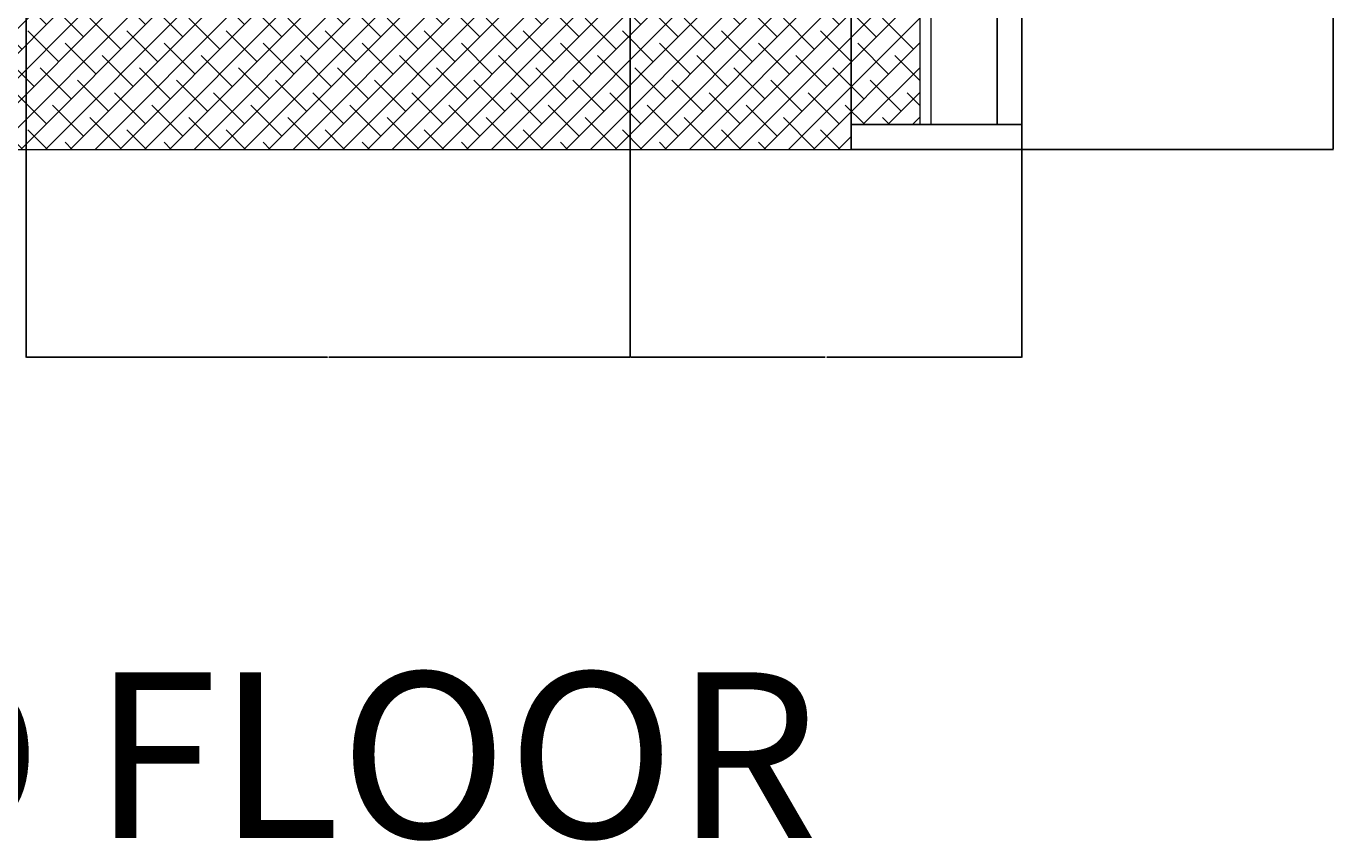
# Model space of a CAD drawing. Units: inches. Extents: x -4843 to -3402, y -164 to 3629.
# Tile 2 of 22: x -4303 to -3829, y -164 to 131. Entities that reach past the tile are written whole.
import ezdxf

# ---------------------------------------------------------------- set-up
doc = ezdxf.new("R2010")
doc.units = ezdxf.units.IN
for name, color, linetype, lineweight in [('A-ANNO-DIMS', 2, 'Continuous', 18), ('A-ANNO-TEXT', 7, 'Continuous', 25), ('C-PROP', 7, 'Continuous', 25), ('C-PVMT', 7, 'Continuous', 18), ('L-PLNT-EDGE', 7, 'Continuous', 18)]:
    doc.layers.add(name, color=color, linetype=linetype, lineweight=lineweight)
doc.layers.add('C-PVMT-PATT', color=9, linetype='Continuous', lineweight=13, true_color=0xc7c8ca)
doc.styles.get("Standard").update_dxf_attribs({"font": 'arial.ttf'})
doc.dimstyles.get("Standard").update_dxf_attribs({"dimtxt": 0.18, "dimasz": 0.18, "dimexe": 0.18, "dimexo": 0.0625, "dimgap": 0.09, "dimtad": 0, "dimtih": 1, "dimtoh": 1, "dimdec": 4, "dimzin": 0, "dimdsep": 46, "dimtxsty": 'Standard', "dimcen": 0.09, "dimadec": 0, "dimazin": 0, "dimtfac": 1, "dimtdec": 4, "dimtofl": 0, "dimtmove": 0, "dimatfit": 3, "dimfxl": 1, "dimtolj": 1, "dimtzin": 0, "dimarcsym": 0})

# ---------------------------------------------------------------- blocks, each defined once
blk = doc.blocks.new('*D61')
at = {"layer": 'A-ANNO-DIMS', "color": 0, "lineweight": -2, "transparency": 16777216}
for p, q in [((-3941.72, 1149.35), (-3828.78, 1149.35)), ((-3828.96, 1149.17), (-3828.96, 618.04)), ((-3828.96, 86.53), (-3828.96, 617.67)), ((-3941.72, 86.35), (-3828.78, 86.35))]:
    blk.add_line(p, q, dxfattribs=at)
at = {"layer": 'A-ANNO-DIMS', "color": 0, "transparency": 16777216}
for points in [[(-3828.99, 1149.17), (-3828.93, 1149.17), (-3828.96, 1149.35)], [(-3828.99, 86.53), (-3828.93, 86.53), (-3828.96, 86.35)]]:
    blk.add_solid(points, dxfattribs=at)
at = {"layer": 'Defpoints', "color": 0, "transparency": 16777216}
for p in [(-3941.78, 1149.35), (-3828.96, 1149.35), (-3941.78, 86.35)]:
    blk.add_point(p, dxfattribs=at)
at = {"layer": 'A-ANNO-DIMS', "color": 0, "transparency": 16777216, "insert": (-3828.96, 617.85), "char_height": 0.18, "attachment_point": 5}
blk.add_mtext('\\A1;1063', dxfattribs=at)
blk = doc.blocks.new('*D63')
at = {"layer": 'A-ANNO-DIMS', "color": 0, "lineweight": -2, "transparency": 16777216}
for p, q in [((-4083.78, 457.29), (-4083.78, 10.92)), ((-4302.78, 275.29), (-4302.78, 10.92)), ((-4302.6, 11.1), (-4193.57, 11.1)), ((-4083.96, 11.1), (-4192.99, 11.1))]:
    blk.add_line(p, q, dxfattribs=at)
at = {"layer": 'A-ANNO-DIMS', "color": 0, "transparency": 16777216}
for points in [[(-4302.6, 11.13), (-4302.6, 11.07), (-4302.78, 11.1)], [(-4083.96, 11.13), (-4083.96, 11.07), (-4083.78, 11.1)]]:
    blk.add_solid(points, dxfattribs=at)
at = {"layer": 'Defpoints', "color": 0, "transparency": 16777216}
for p in [(-4083.78, 457.35), (-4302.78, 275.35), (-4083.78, 11.1)]:
    blk.add_point(p, dxfattribs=at)
at = {"layer": 'A-ANNO-DIMS', "color": 0, "transparency": 16777216, "insert": (-4193.28, 11.1), "char_height": 0.18, "attachment_point": 5}
blk.add_mtext('\\A1;219', dxfattribs=at)
blk = doc.blocks.new('*D66')
at = {"layer": 'A-ANNO-DIMS', "color": 0, "lineweight": -2, "transparency": 16777216}
for p, q in [((-4083.78, 457.29), (-4083.78, 10.92)), ((-3941.78, 86.29), (-3941.78, 10.92)), ((-4083.6, 11.1), (-4013.06, 11.1)), ((-3941.96, 11.1), (-4012.5, 11.1))]:
    blk.add_line(p, q, dxfattribs=at)
at = {"layer": 'A-ANNO-DIMS', "color": 0, "transparency": 16777216}
for points in [[(-4083.6, 11.13), (-4083.6, 11.07), (-4083.78, 11.1)], [(-3941.96, 11.13), (-3941.96, 11.07), (-3941.78, 11.1)]]:
    blk.add_solid(points, dxfattribs=at)
at = {"layer": 'Defpoints', "color": 0, "transparency": 16777216}
for p in [(-4083.78, 457.35), (-3941.78, 86.35), (-3941.78, 11.1)]:
    blk.add_point(p, dxfattribs=at)
at = {"layer": 'A-ANNO-DIMS', "color": 0, "transparency": 16777216, "insert": (-4012.78, 11.1), "char_height": 0.18, "attachment_point": 5}
blk.add_mtext('\\A1;142', dxfattribs=at)
blk = doc.blocks.new('*D81')
at = {"layer": 'A-ANNO-DIMS', "color": 0, "lineweight": -2, "transparency": 16777216}
for p, q in [((-4332.78, 86.42), (-4332.78, 1392.95)), ((-4332.6, 1392.77), (-4168.61, 1392.77)), ((-4003.86, 1392.77), (-4167.86, 1392.77)), ((-4003.68, 86.42), (-4003.68, 1392.95))]:
    blk.add_line(p, q, dxfattribs=at)
at = {"layer": 'A-ANNO-DIMS', "color": 0, "transparency": 16777216}
for points in [[(-4332.6, 1392.8), (-4332.6, 1392.74), (-4332.78, 1392.77)], [(-4003.86, 1392.8), (-4003.86, 1392.74), (-4003.68, 1392.77)]]:
    blk.add_solid(points, dxfattribs=at)
at = {"layer": 'Defpoints', "color": 0, "transparency": 16777216}
for p in [(-4003.68, 1392.77), (-4332.78, 86.35), (-4003.68, 86.35)]:
    blk.add_point(p, dxfattribs=at)
at = {"layer": 'A-ANNO-DIMS', "color": 0, "transparency": 16777216, "insert": (-4168.23, 1392.77), "char_height": 0.18, "attachment_point": 5}
blk.add_mtext('\\A1;329.1', dxfattribs=at)

msp = doc.modelspace()

# ---------------------------------------------------------------- hatches: boundary and pattern name
at = {"layer": 'C-PVMT-PATT'}
h = msp.add_hatch(dxfattribs=at)
h.set_pattern_fill('ANSI38', color=256, scale=2)
h.set_pattern_definition([(45, (-7766.296, -1992.247), (-4.490128, 4.490128), []), (135, (-7766.296, -1992.247), (-13.470384, 4.490128), [15.875, -9.525])])
h.paths.add_polyline_path([(-4583.98, 275.35), (-4595.78, 275.35), (-4595.78, 324.35), (-4595.78, 373.35), (-4595.78, 466.35), (-4696.78, 466.35), (-4696.78, 95.35), (-4583.98, 95.35), (-4583.98, 226.6)])
h.paths.add_polyline_path([(-4302.78, 226.6), (-4583.98, 226.6), (-4583.98, 95.35), (-4332.78, 95.35), (-4332.78, 86.35), (-4003.68, 86.35), (-4003.68, 95.35), (-3978.78, 95.35), (-3978.78, 457.35), (-4003.68, 457.35), (-4003.68, 139.54), (-4302.78, 139.54)])

# ---------------------------------------------------------------- linework, layer by layer
at = {"layer": 'C-PROP'}
for p, q in [((-3941.78, 1149.35), (-3941.78, 86.35)), ((-3950.78, 1140.35), (-3950.78, 95.35)), ((-4003.68, 95.35), (-4003.68, 86.35)), ((-4003.68, 95.35), (-3941.78, 95.35)), ((-3941.78, 86.35), (-4003.68, 86.35))]:
    msp.add_line(p, q, dxfattribs=at)
at = {"layer": 'C-PVMT'}
msp.add_line((-4332.78, 86.35), (-4003.68, 86.35), dxfattribs=at)
at = {"layer": 'L-PLNT-EDGE'}
for p, q in [((-3974.78, 1116.35), (-3974.78, 95.35)), ((-3978.78, 1112.35), (-3978.78, 95.35))]:
    msp.add_line(p, q, dxfattribs=at)

# ---------------------------------------------------------------- texts
at = {"layer": 'A-ANNO-TEXT'}
msp.add_text('GROUND FLOOR', height=60, dxfattribs=at).set_placement((-4640.63, -163.06))

# ---------------------------------------------------------------- dimensions: what is measured, and where the dimension line sits
at = {"layer": 'A-ANNO-DIMS'}
for base, p1, p2, override, picture, middle in [((-4003.68, 1392.77), (-4332.78, 86.35), (-4003.68, 86.35), {"dimdec": 1, "dimlfac": 1, "dimrnd": 0, "dimzin": 0, "dimdsep": 46, "dimlunit": 2}, '*D81', (-4168.23, 1392.77)), ((-4083.78, 11.1), (-4302.78, 275.35), (-4083.78, 457.35), {"dimdec": 0, "dimlfac": 1, "dimrnd": 0, "dimzin": 0, "dimdsep": 46, "dimlunit": 2}, '*D63', (-4193.28, 11.1)), ((-3941.78, 11.1), (-4083.78, 457.35), (-3941.78, 86.35), {"dimdec": 0, "dimlfac": 1, "dimrnd": 0, "dimzin": 0, "dimdsep": 46, "dimlunit": 2}, '*D66', (-4012.78, 11.1))]:
    dim = msp.add_linear_dim(base=base, p1=p1, p2=p2, dimstyle='Standard', override=override, dxfattribs=at)
    dim.commit()
    dim.dimension.update_dxf_attribs({"geometry": picture, "text_midpoint": middle})
dim = msp.add_linear_dim(base=(-3828.96, 1149.35), p1=(-3941.78, 86.35), p2=(-3941.78, 1149.35), angle=90, dimstyle='Standard', override={"dimdec": 0, "dimlfac": 1, "dimrnd": 0, "dimzin": 0, "dimdsep": 46, "dimlunit": 2}, dxfattribs=at)
dim.commit()
dim.dimension.update_dxf_attribs({"geometry": '*D61', "text_midpoint": (-3828.96, 617.85)})

doc.saveas('drawing.dxf')
